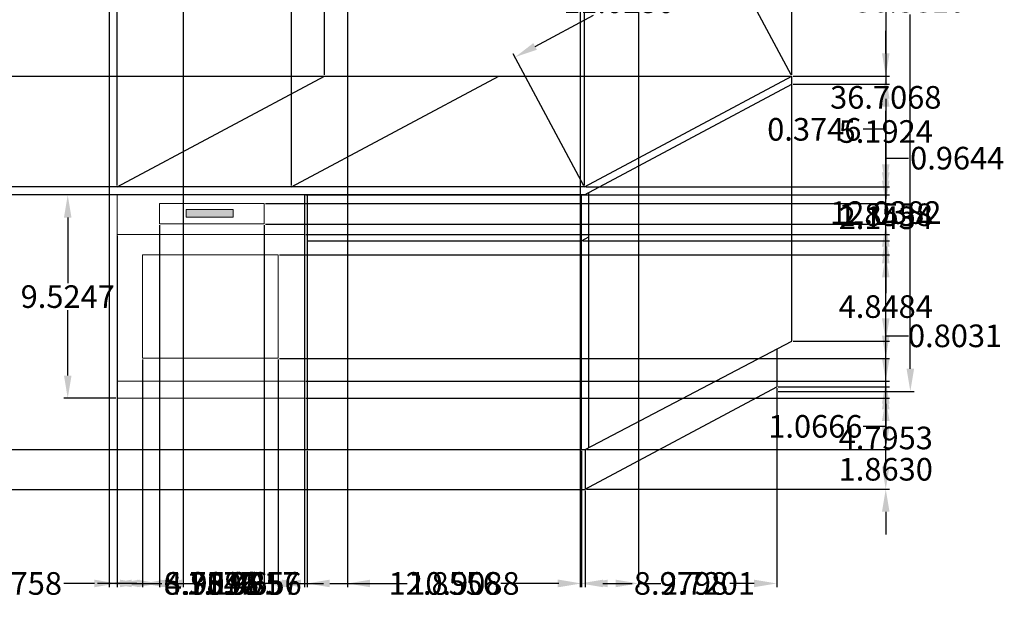
# Model space of a CAD drawing. Units: inches. Extents: x 32.3 to 119.3, y 11.9 to 64.
# Tile 2 of 3: x 73.2 to 119.3, y 11.9 to 39. Entities that reach past the tile are written whole.
import ezdxf

# ---------------------------------------------------------------- set-up
doc = ezdxf.new("R2010")
doc.units = ezdxf.units.IN
doc.header["$MEASUREMENT"] = 0
for name, color, linetype, lineweight in [('A-ANNO-DIMS', 2, 'Continuous', 18), ('A-EQPM', 4, 'Continuous', 18), ('A-EQPM-PATT', 8, 'Continuous', 13), ('A-FURN', 7, 'Continuous', 25)]:
    doc.layers.add(name, color=color, linetype=linetype, lineweight=lineweight)
doc.styles.get("Standard").update_dxf_attribs({"font": 'arial.ttf'})
doc.dimstyles.get("Standard").update_dxf_attribs({"dimtxt": 1.06, "dimasz": 1.06, "dimexe": 0.18, "dimexo": 0.0625, "dimgap": 0.09, "dimtad": 0, "dimtih": 1, "dimtoh": 1, "dimdec": 4, "dimzin": 0, "dimdsep": 46, "dimtxsty": 'Standard', "dimcen": 0.09, "dimadec": 0, "dimazin": 0, "dimtfac": 1, "dimtdec": 4, "dimtofl": 0, "dimtmove": 0, "dimatfit": 3, "dimfxl": 1, "dimtolj": 1, "dimtzin": 0, "dimarcsym": 0})

# ---------------------------------------------------------------- blocks, each defined once
blk = doc.blocks.new('*D8')
at = {"layer": 'A-ANNO-DIMS', "color": 0, "lineweight": -2, "transparency": 16777216}
for p, q in [((77.664, 30.769), (75.233, 30.769)), ((75.413, 29.709), (75.413, 26.637)), ((75.413, 22.304), (75.413, 25.375)), ((77.664, 21.244), (75.233, 21.244))]:
    blk.add_line(p, q, dxfattribs=at)
at = {"layer": 'A-ANNO-DIMS', "color": 0, "transparency": 16777216}
for points in [[(75.237, 29.709), (75.59, 29.709), (75.413, 30.769)], [(75.237, 22.304), (75.59, 22.304), (75.413, 21.244)]]:
    blk.add_solid(points, dxfattribs=at)
at = {"layer": 'Defpoints', "color": 0, "transparency": 16777216}
for p in [(75.413, 30.769), (77.726, 30.769), (77.726, 21.244)]:
    blk.add_point(p, dxfattribs=at)
at = {"layer": 'A-ANNO-DIMS', "color": 0, "transparency": 16777216, "insert": (75.413, 26.006), "char_height": 1.06, "attachment_point": 5}
blk.add_mtext('\\A1;9.5247', dxfattribs=at)
blk = doc.blocks.new('*D10')
at = {"layer": 'A-ANNO-DIMS', "color": 0, "lineweight": -2, "transparency": 16777216}
for p, q in [((109.325, 36.391), (106.022, 42.576)), ((105.172, 41.918), (102.428, 40.453)), ((97.318, 37.724), (100.062, 39.19)), ((99.602, 31.198), (96.298, 37.384))]:
    blk.add_line(p, q, dxfattribs=at)
at = {"layer": 'A-ANNO-DIMS', "color": 0, "transparency": 16777216}
for points in [[(105.088, 42.074), (105.255, 41.762), (106.107, 42.418)], [(97.235, 37.88), (97.401, 37.569), (96.383, 37.225)]]:
    blk.add_solid(points, dxfattribs=at)
at = {"layer": 'Defpoints', "color": 0, "transparency": 16777216}
for p in [(106.107, 42.418), (109.354, 36.335), (99.631, 31.143)]:
    blk.add_point(p, dxfattribs=at)
at = {"layer": 'A-ANNO-DIMS', "color": 0, "transparency": 16777216, "insert": (101.245, 39.821), "char_height": 1.06, "attachment_point": 5}
blk.add_mtext('\\A1;11.0230', dxfattribs=at)
blk = doc.blocks.new('*D11')
at = {"layer": 'A-ANNO-DIMS', "color": 0, "lineweight": -2, "transparency": 16777216}
for p, q in [((108.706, 58.146), (115.085, 58.146)), ((114.905, 57.086), (114.905, 40.487)), ((114.905, 22.625), (114.905, 39.223)), ((108.706, 21.565), (115.085, 21.565))]:
    blk.add_line(p, q, dxfattribs=at)
at = {"layer": 'A-ANNO-DIMS', "color": 0, "transparency": 16777216}
for points in [[(114.729, 57.086), (115.082, 57.086), (114.905, 58.146)], [(114.729, 22.625), (115.082, 22.625), (114.905, 21.565)]]:
    blk.add_solid(points, dxfattribs=at)
at = {"layer": 'Defpoints', "color": 0, "transparency": 16777216}
for p in [(108.644, 58.146), (114.905, 58.146), (108.644, 21.565)]:
    blk.add_point(p, dxfattribs=at)
at = {"layer": 'A-ANNO-DIMS', "color": 0, "transparency": 16777216, "insert": (114.905, 39.855), "char_height": 1.06, "attachment_point": 5}
blk.add_mtext('\\A1;36.5810', dxfattribs=at)
blk = doc.blocks.new('*D12')
at = {"layer": 'A-ANNO-DIMS', "color": 0, "lineweight": -2, "transparency": 16777216}
for p, q in [((42.508, 51.967), (42.508, 58.272)), ((109.354, 36.398), (109.354, 58.272)), ((43.568, 58.092), (73.222, 58.092)), ((108.294, 58.092), (78.64, 58.092))]:
    blk.add_line(p, q, dxfattribs=at)
at = {"layer": 'A-ANNO-DIMS', "color": 0, "transparency": 16777216}
for points in [[(43.568, 58.269), (43.568, 57.916), (42.508, 58.092)], [(108.294, 58.269), (108.294, 57.916), (109.354, 58.092)]]:
    blk.add_solid(points, dxfattribs=at)
at = {"layer": 'Defpoints', "color": 0, "transparency": 16777216}
for p in [(109.354, 58.092), (42.508, 51.905), (109.354, 36.335)]:
    blk.add_point(p, dxfattribs=at)
at = {"layer": 'A-ANNO-DIMS', "color": 0, "transparency": 16777216, "insert": (75.931, 58.092), "char_height": 1.06, "attachment_point": 5}
blk.add_mtext('\\A1;66.8465', dxfattribs=at)
blk = doc.blocks.new('*D16')
at = {"layer": 'A-ANNO-DIMS', "color": 0, "lineweight": -2, "transparency": 16777216}
for p, q in [((77.726, 21.181), (77.726, 12.388)), ((68.15, 18.786), (68.15, 12.388)), ((69.21, 12.568), (70.647, 12.568)), ((76.666, 12.568), (75.23, 12.568))]:
    blk.add_line(p, q, dxfattribs=at)
at = {"layer": 'A-ANNO-DIMS', "color": 0, "transparency": 16777216}
for points in [[(69.21, 12.745), (69.21, 12.391), (68.15, 12.568)], [(76.666, 12.745), (76.666, 12.391), (77.726, 12.568)]]:
    blk.add_solid(points, dxfattribs=at)
at = {"layer": 'Defpoints', "color": 0, "transparency": 16777216}
for p in [(77.726, 21.244), (68.15, 18.849), (77.726, 12.568)]:
    blk.add_point(p, dxfattribs=at)
at = {"layer": 'A-ANNO-DIMS', "color": 0, "transparency": 16777216, "insert": (72.938, 12.568), "char_height": 1.06, "attachment_point": 5}
blk.add_mtext('\\A1;9.5758', dxfattribs=at)
blk = doc.blocks.new('*D17')
at = {"layer": 'A-ANNO-DIMS', "color": 0, "lineweight": -2, "transparency": 16777216}
for p, q in [((77.726, 21.181), (77.726, 12.388)), ((86.511, 21.181), (86.511, 12.388)), ((78.786, 12.568), (79.828, 12.568)), ((85.451, 12.568), (84.409, 12.568))]:
    blk.add_line(p, q, dxfattribs=at)
at = {"layer": 'A-ANNO-DIMS', "color": 0, "transparency": 16777216}
for points in [[(78.786, 12.745), (78.786, 12.391), (77.726, 12.568)], [(85.451, 12.745), (85.451, 12.391), (86.511, 12.568)]]:
    blk.add_solid(points, dxfattribs=at)
at = {"layer": 'Defpoints', "color": 0, "transparency": 16777216}
for p in [(77.726, 21.244), (86.511, 21.244), (86.511, 12.568)]:
    blk.add_point(p, dxfattribs=at)
at = {"layer": 'A-ANNO-DIMS', "color": 0, "transparency": 16777216, "insert": (82.119, 12.568), "char_height": 1.06, "attachment_point": 5}
blk.add_mtext('\\A1;8.7846', dxfattribs=at)
blk = doc.blocks.new('*D18')
at = {"layer": 'A-ANNO-DIMS', "color": 0, "lineweight": -2, "transparency": 16777216}
for p, q in [((86.634, 18.786), (86.634, 12.388)), ((99.489, 18.786), (99.489, 12.388)), ((87.694, 12.568), (90.41, 12.568)), ((98.429, 12.568), (95.713, 12.568))]:
    blk.add_line(p, q, dxfattribs=at)
at = {"layer": 'A-ANNO-DIMS', "color": 0, "transparency": 16777216}
for points in [[(87.694, 12.745), (87.694, 12.391), (86.634, 12.568)], [(98.429, 12.745), (98.429, 12.391), (99.489, 12.568)]]:
    blk.add_solid(points, dxfattribs=at)
at = {"layer": 'Defpoints', "color": 0, "transparency": 16777216}
for p in [(86.634, 18.849), (99.489, 18.849), (99.489, 12.568)]:
    blk.add_point(p, dxfattribs=at)
at = {"layer": 'A-ANNO-DIMS', "color": 0, "transparency": 16777216, "insert": (93.062, 12.568), "char_height": 1.06, "attachment_point": 5}
blk.add_mtext('\\A1;12.8556', dxfattribs=at)
blk = doc.blocks.new('*D19')
at = {"layer": 'A-ANNO-DIMS', "color": 0, "lineweight": -2, "transparency": 16777216}
for p, q in [((108.644, 21.718), (108.644, 12.388)), ((99.664, 16.923), (99.664, 12.388)), ((100.724, 12.568), (101.862, 12.568)), ((107.584, 12.568), (106.446, 12.568))]:
    blk.add_line(p, q, dxfattribs=at)
at = {"layer": 'A-ANNO-DIMS', "color": 0, "transparency": 16777216}
for points in [[(100.724, 12.745), (100.724, 12.391), (99.664, 12.568)], [(107.584, 12.745), (107.584, 12.391), (108.644, 12.568)]]:
    blk.add_solid(points, dxfattribs=at)
at = {"layer": 'Defpoints', "color": 0, "transparency": 16777216}
for p in [(108.644, 21.781), (99.664, 16.986), (108.644, 12.568)]:
    blk.add_point(p, dxfattribs=at)
at = {"layer": 'A-ANNO-DIMS', "color": 0, "transparency": 16777216, "insert": (104.154, 12.568), "char_height": 1.06, "attachment_point": 5}
blk.add_mtext('\\A1;8.9798', dxfattribs=at)
blk = doc.blocks.new('*D20')
at = {"layer": 'A-ANNO-DIMS', "color": 0, "lineweight": -2, "transparency": 16777216}
for p, q in [((108.706, 21.781), (113.934, 21.781)), ((113.754, 20.721), (113.754, 20.015)), ((113.754, 18.046), (113.754, 18.752)), ((99.726, 16.986), (113.934, 16.986))]:
    blk.add_line(p, q, dxfattribs=at)
at = {"layer": 'A-ANNO-DIMS', "color": 0, "transparency": 16777216}
for points in [[(113.578, 20.721), (113.931, 20.721), (113.754, 21.781)], [(113.578, 18.046), (113.931, 18.046), (113.754, 16.986)]]:
    blk.add_solid(points, dxfattribs=at)
at = {"layer": 'Defpoints', "color": 0, "transparency": 16777216}
for p in [(108.644, 21.781), (113.754, 21.781), (99.664, 16.986)]:
    blk.add_point(p, dxfattribs=at)
at = {"layer": 'A-ANNO-DIMS', "color": 0, "transparency": 16777216, "insert": (113.754, 19.383), "char_height": 1.06, "attachment_point": 5}
blk.add_mtext('\\A1;4.7953', dxfattribs=at)
blk = doc.blocks.new('*D21')
at = {"layer": 'A-ANNO-DIMS', "color": 0, "lineweight": -2, "transparency": 16777216}
for p, q in [((113.754, 19.909), (113.754, 20.969)), ((99.727, 18.849), (113.934, 18.849)), ((99.726, 16.986), (113.934, 16.986)), ((113.754, 15.926), (113.754, 14.866))]:
    blk.add_line(p, q, dxfattribs=at)
at = {"layer": 'A-ANNO-DIMS', "color": 0, "transparency": 16777216}
for points in [[(113.578, 19.909), (113.931, 19.909), (113.754, 18.849)], [(113.578, 15.926), (113.931, 15.926), (113.754, 16.986)]]:
    blk.add_solid(points, dxfattribs=at)
at = {"layer": 'Defpoints', "color": 0, "transparency": 16777216}
for p in [(99.664, 18.849), (113.754, 18.849), (99.664, 16.986)]:
    blk.add_point(p, dxfattribs=at)
at = {"layer": 'A-ANNO-DIMS', "color": 0, "transparency": 16777216, "insert": (113.754, 17.917), "char_height": 1.06, "attachment_point": 5}
blk.add_mtext('\\A1;1.8630', dxfattribs=at)
blk = doc.blocks.new('*D22')
at = {"layer": 'A-ANNO-DIMS', "color": 0, "lineweight": -2, "transparency": 16777216}
for p, q in [((109.417, 35.961), (113.934, 35.961)), ((113.754, 34.901), (113.754, 30.573)), ((113.754, 24.983), (113.754, 29.31)), ((109.417, 23.923), (113.934, 23.923))]:
    blk.add_line(p, q, dxfattribs=at)
at = {"layer": 'A-ANNO-DIMS', "color": 0, "transparency": 16777216}
for points in [[(113.578, 34.901), (113.931, 34.901), (113.754, 35.961)], [(113.578, 24.983), (113.931, 24.983), (113.754, 23.923)]]:
    blk.add_solid(points, dxfattribs=at)
at = {"layer": 'Defpoints', "color": 0, "transparency": 16777216}
for p in [(109.354, 35.961), (113.754, 35.961), (109.354, 23.923)]:
    blk.add_point(p, dxfattribs=at)
at = {"layer": 'A-ANNO-DIMS', "color": 0, "transparency": 16777216, "insert": (113.754, 29.942), "char_height": 1.06, "attachment_point": 5}
blk.add_mtext('\\A1;12.0382', dxfattribs=at)
blk = doc.blocks.new('*D23')
at = {"layer": 'A-ANNO-DIMS', "color": 0, "lineweight": -2, "transparency": 16777216}
for p, q in [((102.22, 53.692), (113.934, 53.692)), ((113.754, 52.632), (113.754, 35.971)), ((113.754, 18.046), (113.754, 34.708)), ((99.726, 16.986), (113.934, 16.986))]:
    blk.add_line(p, q, dxfattribs=at)
at = {"layer": 'A-ANNO-DIMS', "color": 0, "transparency": 16777216}
for points in [[(113.578, 52.632), (113.931, 52.632), (113.754, 53.692)], [(113.578, 18.046), (113.931, 18.046), (113.754, 16.986)]]:
    blk.add_solid(points, dxfattribs=at)
at = {"layer": 'Defpoints', "color": 0, "transparency": 16777216}
for p in [(102.157, 53.692), (113.754, 53.692), (99.664, 16.986)]:
    blk.add_point(p, dxfattribs=at)
at = {"layer": 'A-ANNO-DIMS', "color": 0, "transparency": 16777216, "insert": (113.754, 35.339), "char_height": 1.06, "attachment_point": 5}
blk.add_mtext('\\A1;36.7068', dxfattribs=at)
blk = doc.blocks.new('*D27')
at = {"layer": 'A-ANNO-DIMS', "color": 0, "lineweight": -2, "transparency": 16777216}
for p, q in [((88.528, 44.465), (88.528, 12.388)), ((99.437, 44.465), (99.437, 12.388)), ((89.588, 12.568), (91.33, 12.568)), ((98.377, 12.568), (96.636, 12.568))]:
    blk.add_line(p, q, dxfattribs=at)
at = {"layer": 'A-ANNO-DIMS', "color": 0, "transparency": 16777216}
for points in [[(89.588, 12.745), (89.588, 12.391), (88.528, 12.568)], [(98.377, 12.745), (98.377, 12.391), (99.437, 12.568)]]:
    blk.add_solid(points, dxfattribs=at)
at = {"layer": 'Defpoints', "color": 0, "transparency": 16777216}
for p in [(88.528, 44.527), (99.437, 44.527), (99.437, 12.568)]:
    blk.add_point(p, dxfattribs=at)
at = {"layer": 'A-ANNO-DIMS', "color": 0, "transparency": 16777216, "insert": (93.983, 12.568), "char_height": 1.06, "attachment_point": 5}
blk.add_mtext('\\A1;10.9088', dxfattribs=at)
blk = doc.blocks.new('*D28')
at = {"layer": 'A-ANNO-DIMS', "color": 0, "lineweight": -2, "transparency": 16777216}
for p, q in [((102.157, 44.957), (102.157, 12.388)), ((99.437, 44.465), (99.437, 12.388)), ((100.497, 12.568), (101.097, 12.568)), ((102.157, 12.568), (103.217, 12.568))]:
    blk.add_line(p, q, dxfattribs=at)
at = {"layer": 'A-ANNO-DIMS', "color": 0, "transparency": 16777216}
for points in [[(100.497, 12.745), (100.497, 12.391), (99.437, 12.568)], [(101.097, 12.745), (101.097, 12.391), (102.157, 12.568)]]:
    blk.add_solid(points, dxfattribs=at)
at = {"layer": 'Defpoints', "color": 0, "transparency": 16777216}
for p in [(102.157, 45.02), (99.437, 44.527), (102.157, 12.568)]:
    blk.add_point(p, dxfattribs=at)
at = {"layer": 'A-ANNO-DIMS', "color": 0, "transparency": 16777216, "insert": (105.414, 12.568), "char_height": 1.06, "attachment_point": 5}
blk.add_mtext('\\A1;2.7201', dxfattribs=at)
blk = doc.blocks.new('*D33')
at = {"layer": 'A-ANNO-DIMS', "color": 0, "lineweight": -2, "transparency": 16777216}
for p, q in [((113.754, 31.829), (113.754, 32.889)), ((99.552, 30.769), (113.934, 30.769)), ((99.552, 28.625), (113.934, 28.625)), ((113.754, 27.565), (113.754, 26.505))]:
    blk.add_line(p, q, dxfattribs=at)
at = {"layer": 'A-ANNO-DIMS', "color": 0, "transparency": 16777216}
for points in [[(113.578, 31.829), (113.931, 31.829), (113.754, 30.769)], [(113.578, 27.565), (113.931, 27.565), (113.754, 28.625)]]:
    blk.add_solid(points, dxfattribs=at)
at = {"layer": 'Defpoints', "color": 0, "transparency": 16777216}
for p in [(99.489, 30.769), (113.754, 30.769), (99.489, 28.625)]:
    blk.add_point(p, dxfattribs=at)
at = {"layer": 'A-ANNO-DIMS', "color": 0, "transparency": 16777216, "insert": (113.754, 29.697), "char_height": 1.06, "attachment_point": 5}
blk.add_mtext('\\A1;2.1434', dxfattribs=at)
blk = doc.blocks.new('*D39')
at = {"layer": 'A-ANNO-DIMS', "color": 0, "lineweight": -2, "transparency": 16777216}
for p, q in [((77.355, 44.465), (77.355, 12.388)), ((80.821, 44.632), (80.821, 12.388)), ((78.415, 12.568), (79.761, 12.568)), ((80.821, 12.568), (81.881, 12.568))]:
    blk.add_line(p, q, dxfattribs=at)
at = {"layer": 'A-ANNO-DIMS', "color": 0, "transparency": 16777216}
for points in [[(78.415, 12.745), (78.415, 12.391), (77.355, 12.568)], [(79.761, 12.745), (79.761, 12.391), (80.821, 12.568)]]:
    blk.add_solid(points, dxfattribs=at)
at = {"layer": 'Defpoints', "color": 0, "transparency": 16777216}
for p in [(77.355, 44.527), (80.821, 44.694), (80.821, 12.568)]:
    blk.add_point(p, dxfattribs=at)
at = {"layer": 'A-ANNO-DIMS', "color": 0, "transparency": 16777216, "insert": (84.17, 12.568), "char_height": 1.06, "attachment_point": 5}
blk.add_mtext('\\A1;3.4656', dxfattribs=at)
blk = doc.blocks.new('*D45')
at = {"layer": 'A-ANNO-DIMS', "color": 0, "lineweight": -2, "transparency": 16777216}
for p, q in [((77.725, 31.206), (77.725, 58.272)), ((85.9, 31.206), (85.9, 58.272)), ((78.785, 58.092), (79.521, 58.092)), ((84.84, 58.092), (84.105, 58.092))]:
    blk.add_line(p, q, dxfattribs=at)
at = {"layer": 'A-ANNO-DIMS', "color": 0, "transparency": 16777216}
for points in [[(78.785, 58.269), (78.785, 57.916), (77.725, 58.092)], [(84.84, 58.269), (84.84, 57.916), (85.9, 58.092)]]:
    blk.add_solid(points, dxfattribs=at)
at = {"layer": 'Defpoints', "color": 0, "transparency": 16777216}
for p in [(85.9, 58.092), (77.725, 31.143), (85.9, 31.143)]:
    blk.add_point(p, dxfattribs=at)
at = {"layer": 'A-ANNO-DIMS', "color": 0, "transparency": 16777216, "insert": (81.813, 58.092), "char_height": 1.06, "attachment_point": 5}
blk.add_mtext('\\A1;8.1748', dxfattribs=at)
blk = doc.blocks.new('*D46')
at = {"layer": 'A-ANNO-DIMS', "color": 0, "lineweight": -2, "transparency": 16777216}
for p, q in [((77.725, 31.206), (77.725, 58.272)), ((87.449, 36.398), (87.449, 58.272)), ((78.785, 58.092), (80.293, 58.092)), ((86.389, 58.092), (84.881, 58.092))]:
    blk.add_line(p, q, dxfattribs=at)
at = {"layer": 'A-ANNO-DIMS', "color": 0, "transparency": 16777216}
for points in [[(78.785, 58.269), (78.785, 57.916), (77.725, 58.092)], [(86.389, 58.269), (86.389, 57.916), (87.449, 58.092)]]:
    blk.add_solid(points, dxfattribs=at)
at = {"layer": 'Defpoints', "color": 0, "transparency": 16777216}
for p in [(87.449, 58.092), (87.449, 36.335), (77.725, 31.143)]:
    blk.add_point(p, dxfattribs=at)
at = {"layer": 'A-ANNO-DIMS', "color": 0, "transparency": 16777216, "insert": (82.587, 58.092), "char_height": 1.06, "attachment_point": 5}
blk.add_mtext('\\A1;9.7235', dxfattribs=at)
blk = doc.blocks.new('*D47')
at = {"layer": 'A-ANNO-DIMS', "color": 0, "lineweight": -2, "transparency": 16777216}
for p, q in [((85.9, 31.206), (85.9, 58.272)), ((99.631, 31.206), (99.631, 58.272)), ((86.96, 58.092), (90.115, 58.092)), ((98.571, 58.092), (95.416, 58.092))]:
    blk.add_line(p, q, dxfattribs=at)
at = {"layer": 'A-ANNO-DIMS', "color": 0, "transparency": 16777216}
for points in [[(86.96, 58.269), (86.96, 57.916), (85.9, 58.092)], [(98.571, 58.269), (98.571, 57.916), (99.631, 58.092)]]:
    blk.add_solid(points, dxfattribs=at)
at = {"layer": 'Defpoints', "color": 0, "transparency": 16777216}
for p in [(99.631, 58.092), (85.9, 31.143), (99.631, 31.143)]:
    blk.add_point(p, dxfattribs=at)
at = {"layer": 'A-ANNO-DIMS', "color": 0, "transparency": 16777216, "insert": (92.765, 58.092), "char_height": 1.06, "attachment_point": 5}
blk.add_mtext('\\A1;13.7310', dxfattribs=at)
blk = doc.blocks.new('*D48')
at = {"layer": 'A-ANNO-DIMS', "color": 0, "lineweight": -2, "transparency": 16777216}
for p, q in [((99.631, 31.206), (99.631, 58.272)), ((109.354, 36.398), (109.354, 58.272)), ((100.691, 58.092), (102.198, 58.092)), ((108.294, 58.092), (106.787, 58.092))]:
    blk.add_line(p, q, dxfattribs=at)
at = {"layer": 'A-ANNO-DIMS', "color": 0, "transparency": 16777216}
for points in [[(100.691, 58.269), (100.691, 57.916), (99.631, 58.092)], [(108.294, 58.269), (108.294, 57.916), (109.354, 58.092)]]:
    blk.add_solid(points, dxfattribs=at)
at = {"layer": 'Defpoints', "color": 0, "transparency": 16777216}
for p in [(109.354, 58.092), (109.354, 36.335), (99.631, 31.143)]:
    blk.add_point(p, dxfattribs=at)
at = {"layer": 'A-ANNO-DIMS', "color": 0, "transparency": 16777216, "insert": (104.493, 58.092), "char_height": 1.06, "attachment_point": 5}
blk.add_mtext('\\A1;9.7235', dxfattribs=at)
blk = doc.blocks.new('*D49')
at = {"layer": 'A-ANNO-DIMS', "color": 0, "lineweight": -2, "transparency": 16777216}
for p, q in [((109.417, 36.335), (113.934, 36.335)), ((113.754, 35.275), (113.754, 34.37)), ((113.754, 32.203), (113.754, 33.108)), ((99.693, 31.143), (113.934, 31.143))]:
    blk.add_line(p, q, dxfattribs=at)
at = {"layer": 'A-ANNO-DIMS', "color": 0, "transparency": 16777216}
for points in [[(113.578, 35.275), (113.931, 35.275), (113.754, 36.335)], [(113.578, 32.203), (113.931, 32.203), (113.754, 31.143)]]:
    blk.add_solid(points, dxfattribs=at)
at = {"layer": 'Defpoints', "color": 0, "transparency": 16777216}
for p in [(109.354, 36.335), (113.754, 36.335), (99.631, 31.143)]:
    blk.add_point(p, dxfattribs=at)
at = {"layer": 'A-ANNO-DIMS', "color": 0, "transparency": 16777216, "insert": (113.754, 33.739), "char_height": 1.06, "attachment_point": 5}
blk.add_mtext('\\A1;5.1924', dxfattribs=at)
blk = doc.blocks.new('*D50')
at = {"layer": 'A-ANNO-DIMS', "color": 0, "lineweight": -2, "transparency": 16777216}
for p, q in [((113.754, 37.395), (113.754, 38.455)), ((109.417, 36.335), (113.934, 36.335)), ((109.417, 35.961), (113.934, 35.961)), ((113.754, 34.901), (113.754, 33.841)), ((113.754, 33.841), (112.694, 33.841))]:
    blk.add_line(p, q, dxfattribs=at)
at = {"layer": 'A-ANNO-DIMS', "color": 0, "transparency": 16777216}
for points in [[(113.578, 37.395), (113.931, 37.395), (113.754, 36.335)], [(113.578, 34.901), (113.931, 34.901), (113.754, 35.961)]]:
    blk.add_solid(points, dxfattribs=at)
at = {"layer": 'Defpoints', "color": 0, "transparency": 16777216}
for p in [(109.354, 36.335), (109.354, 35.961), (113.754, 35.961)]:
    blk.add_point(p, dxfattribs=at)
at = {"layer": 'A-ANNO-DIMS', "color": 0, "transparency": 16777216, "insert": (110.405, 33.841), "char_height": 1.06, "attachment_point": 5}
blk.add_mtext('\\A1;0.3746', dxfattribs=at)
blk = doc.blocks.new('*D52')
at = {"layer": 'A-ANNO-DIMS', "color": 0, "lineweight": -2, "transparency": 16777216}
for p, q in [((113.754, 31.829), (113.754, 32.889)), ((86.573, 30.769), (113.934, 30.769)), ((86.573, 28.913), (113.934, 28.913)), ((113.754, 27.853), (113.754, 26.793))]:
    blk.add_line(p, q, dxfattribs=at)
at = {"layer": 'A-ANNO-DIMS', "color": 0, "transparency": 16777216}
for points in [[(113.578, 31.829), (113.931, 31.829), (113.754, 30.769)], [(113.578, 27.853), (113.931, 27.853), (113.754, 28.913)]]:
    blk.add_solid(points, dxfattribs=at)
at = {"layer": 'Defpoints', "color": 0, "transparency": 16777216}
for p in [(86.511, 30.769), (113.754, 30.769), (86.511, 28.913)]:
    blk.add_point(p, dxfattribs=at)
at = {"layer": 'A-ANNO-DIMS', "color": 0, "transparency": 16777216, "insert": (113.754, 29.841), "char_height": 1.06, "attachment_point": 5}
blk.add_mtext('\\A1;1.8558', dxfattribs=at)
blk = doc.blocks.new('*D53')
at = {"layer": 'A-ANNO-DIMS', "color": 0, "lineweight": -2, "transparency": 16777216}
for p, q in [((113.754, 23.107), (113.754, 24.167)), ((113.754, 24.167), (114.814, 24.167)), ((86.573, 22.047), (113.934, 22.047)), ((86.573, 21.244), (113.934, 21.244)), ((113.754, 20.184), (113.754, 19.124))]:
    blk.add_line(p, q, dxfattribs=at)
at = {"layer": 'A-ANNO-DIMS', "color": 0, "transparency": 16777216}
for points in [[(113.578, 23.107), (113.931, 23.107), (113.754, 22.047)], [(113.578, 20.184), (113.931, 20.184), (113.754, 21.244)]]:
    blk.add_solid(points, dxfattribs=at)
at = {"layer": 'Defpoints', "color": 0, "transparency": 16777216}
for p in [(86.511, 22.047), (113.754, 22.047), (86.511, 21.244)]:
    blk.add_point(p, dxfattribs=at)
at = {"layer": 'A-ANNO-DIMS', "color": 0, "transparency": 16777216, "insert": (117.002, 24.167), "char_height": 1.06, "attachment_point": 5}
blk.add_mtext('\\A1;0.8031', dxfattribs=at)
blk = doc.blocks.new('*D54')
at = {"layer": 'A-ANNO-DIMS', "color": 0, "lineweight": -2, "transparency": 16777216}
for p, q in [((79.712, 29.344), (79.712, 12.388)), ((84.622, 29.344), (84.622, 12.388)), ((78.652, 12.568), (77.592, 12.568)), ((85.682, 12.568), (86.742, 12.568))]:
    blk.add_line(p, q, dxfattribs=at)
at = {"layer": 'A-ANNO-DIMS', "color": 0, "transparency": 16777216}
for points in [[(78.652, 12.745), (78.652, 12.391), (79.712, 12.568)], [(85.682, 12.745), (85.682, 12.391), (84.622, 12.568)]]:
    blk.add_solid(points, dxfattribs=at)
at = {"layer": 'Defpoints', "color": 0, "transparency": 16777216}
for p in [(79.712, 29.406), (84.622, 29.406), (84.622, 12.568)]:
    blk.add_point(p, dxfattribs=at)
at = {"layer": 'A-ANNO-DIMS', "color": 0, "transparency": 16777216, "insert": (82.167, 12.568), "char_height": 1.06, "attachment_point": 5}
blk.add_mtext('\\A1;4.9096', dxfattribs=at)
blk = doc.blocks.new('*D55')
at = {"layer": 'A-ANNO-DIMS', "color": 0, "lineweight": -2, "transparency": 16777216}
for p, q in [((113.754, 31.431), (113.754, 32.491)), ((113.754, 32.491), (114.814, 32.491)), ((84.684, 30.371), (113.934, 30.371)), ((84.684, 29.406), (113.934, 29.406)), ((113.754, 28.346), (113.754, 27.286))]:
    blk.add_line(p, q, dxfattribs=at)
at = {"layer": 'A-ANNO-DIMS', "color": 0, "transparency": 16777216}
for points in [[(113.578, 31.431), (113.931, 31.431), (113.754, 30.371)], [(113.578, 28.346), (113.931, 28.346), (113.754, 29.406)]]:
    blk.add_solid(points, dxfattribs=at)
at = {"layer": 'Defpoints', "color": 0, "transparency": 16777216}
for p in [(84.622, 30.371), (113.754, 30.371), (84.622, 29.406)]:
    blk.add_point(p, dxfattribs=at)
at = {"layer": 'A-ANNO-DIMS', "color": 0, "transparency": 16777216, "insert": (117.103, 32.491), "char_height": 1.06, "attachment_point": 5}
blk.add_mtext('\\A1;0.9644', dxfattribs=at)
blk = doc.blocks.new('*D56')
at = {"layer": 'A-ANNO-DIMS', "color": 0, "lineweight": -2, "transparency": 16777216}
for p, q in [((79.712, 29.344), (79.712, 12.388)), ((77.726, 28.85), (77.726, 12.388)), ((76.666, 12.568), (75.606, 12.568)), ((80.772, 12.568), (81.832, 12.568))]:
    blk.add_line(p, q, dxfattribs=at)
at = {"layer": 'A-ANNO-DIMS', "color": 0, "transparency": 16777216}
for points in [[(76.666, 12.745), (76.666, 12.391), (77.726, 12.568)], [(80.772, 12.745), (80.772, 12.391), (79.712, 12.568)]]:
    blk.add_solid(points, dxfattribs=at)
at = {"layer": 'Defpoints', "color": 0, "transparency": 16777216}
for p in [(79.712, 29.406), (77.726, 28.913), (79.712, 12.568)]:
    blk.add_point(p, dxfattribs=at)
at = {"layer": 'A-ANNO-DIMS', "color": 0, "transparency": 16777216, "insert": (84.072, 12.568), "char_height": 1.06, "attachment_point": 5}
blk.add_mtext('\\A1;1.9857', dxfattribs=at)
blk = doc.blocks.new('*D57')
at = {"layer": 'A-ANNO-DIMS', "color": 0, "lineweight": -2, "transparency": 16777216}
for p, q in [((78.925, 23.051), (78.925, 12.388)), ((85.283, 23.051), (85.283, 12.388)), ((77.865, 12.568), (76.805, 12.568)), ((86.343, 12.568), (87.403, 12.568))]:
    blk.add_line(p, q, dxfattribs=at)
at = {"layer": 'A-ANNO-DIMS', "color": 0, "transparency": 16777216}
for points in [[(77.865, 12.745), (77.865, 12.391), (78.925, 12.568)], [(86.343, 12.745), (86.343, 12.391), (85.283, 12.568)]]:
    blk.add_solid(points, dxfattribs=at)
at = {"layer": 'Defpoints', "color": 0, "transparency": 16777216}
for p in [(78.925, 23.113), (85.283, 23.113), (85.283, 12.568)]:
    blk.add_point(p, dxfattribs=at)
at = {"layer": 'A-ANNO-DIMS', "color": 0, "transparency": 16777216, "insert": (82.104, 12.568), "char_height": 1.06, "attachment_point": 5}
blk.add_mtext('\\A1;6.3577', dxfattribs=at)
blk = doc.blocks.new('*D58')
at = {"layer": 'A-ANNO-DIMS', "color": 0, "lineweight": -2, "transparency": 16777216}
for p, q in [((85.346, 27.962), (113.934, 27.962)), ((113.754, 26.902), (113.754, 26.169)), ((113.754, 24.173), (113.754, 24.906)), ((85.346, 23.113), (113.934, 23.113))]:
    blk.add_line(p, q, dxfattribs=at)
at = {"layer": 'A-ANNO-DIMS', "color": 0, "transparency": 16777216}
for points in [[(113.578, 26.902), (113.931, 26.902), (113.754, 27.962)], [(113.578, 24.173), (113.931, 24.173), (113.754, 23.113)]]:
    blk.add_solid(points, dxfattribs=at)
at = {"layer": 'Defpoints', "color": 0, "transparency": 16777216}
for p in [(85.283, 27.962), (113.754, 27.962), (85.283, 23.113)]:
    blk.add_point(p, dxfattribs=at)
at = {"layer": 'A-ANNO-DIMS', "color": 0, "transparency": 16777216, "insert": (113.754, 25.538), "char_height": 1.06, "attachment_point": 5}
blk.add_mtext('\\A1;4.8484', dxfattribs=at)
blk = doc.blocks.new('*D59')
at = {"layer": 'A-ANNO-DIMS', "color": 0, "lineweight": -2, "transparency": 16777216}
for p, q in [((78.925, 23.051), (78.925, 12.388)), ((77.726, 21.984), (77.726, 12.388)), ((76.666, 12.568), (75.606, 12.568)), ((79.985, 12.568), (81.045, 12.568))]:
    blk.add_line(p, q, dxfattribs=at)
at = {"layer": 'A-ANNO-DIMS', "color": 0, "transparency": 16777216}
for points in [[(76.666, 12.745), (76.666, 12.391), (77.726, 12.568)], [(79.985, 12.745), (79.985, 12.391), (78.925, 12.568)]]:
    blk.add_solid(points, dxfattribs=at)
at = {"layer": 'Defpoints', "color": 0, "transparency": 16777216}
for p in [(78.925, 23.113), (77.726, 22.047), (78.925, 12.568)]:
    blk.add_point(p, dxfattribs=at)
at = {"layer": 'A-ANNO-DIMS', "color": 0, "transparency": 16777216, "insert": (83.183, 12.568), "char_height": 1.06, "attachment_point": 5}
blk.add_mtext('\\A1;1.1991', dxfattribs=at)
blk = doc.blocks.new('*D60')
at = {"layer": 'A-ANNO-DIMS', "color": 0, "lineweight": -2, "transparency": 16777216}
for p, q in [((113.754, 24.173), (113.754, 25.233)), ((85.346, 23.113), (113.934, 23.113)), ((86.573, 22.047), (113.934, 22.047)), ((113.754, 20.987), (113.754, 19.927)), ((113.754, 19.927), (112.694, 19.927))]:
    blk.add_line(p, q, dxfattribs=at)
at = {"layer": 'A-ANNO-DIMS', "color": 0, "transparency": 16777216}
for points in [[(113.578, 24.173), (113.931, 24.173), (113.754, 23.113)], [(113.578, 20.987), (113.931, 20.987), (113.754, 22.047)]]:
    blk.add_solid(points, dxfattribs=at)
at = {"layer": 'Defpoints', "color": 0, "transparency": 16777216}
for p in [(85.283, 23.113), (86.511, 22.047), (113.754, 22.047)]:
    blk.add_point(p, dxfattribs=at)
at = {"layer": 'A-ANNO-DIMS', "color": 0, "transparency": 16777216, "insert": (110.454, 19.927), "char_height": 1.06, "attachment_point": 5}
blk.add_mtext('\\A1;1.0666', dxfattribs=at)

msp = doc.modelspace()

# ---------------------------------------------------------------- hatches: boundary and pattern name
at = {"layer": 'A-EQPM-PATT'}
h = msp.add_hatch(color=256, dxfattribs=at)
h.dxf.hatch_style = 1
h.paths.add_polyline_path([(83.17165, 30.07967), (80.9625, 30.07967), (80.9625, 29.73156), (83.17165, 29.73156)])

# ---------------------------------------------------------------- linework, layer by layer
at = {"layer": 'A-EQPM'}
for p, q in [((77.72624, 30.76852), (77.72624, 21.24379)), ((77.72624, 28.91269), (86.51084, 28.91269)), ((77.72624, 22.04688), (86.51084, 22.04688)), ((77.72624, 21.24379), (86.51084, 21.24379))]:
    msp.add_line(p, q, dxfattribs=at)
for points in [[(79.71198, 30.37063), (84.62155, 30.37063), (84.62155, 29.4062), (79.71198, 29.4062)], [(80.9625, 30.07967), (83.17165, 30.07967), (83.17165, 29.73156), (80.9625, 29.73156)], [(78.9253, 27.96182), (85.283, 27.96182), (85.283, 23.11347), (78.9253, 23.11347)]]:
    msp.add_lwpolyline(points, close=True, dxfattribs=at)
at = {"layer": 'A-FURN'}
for p, q in [((63.93986, 36.33549), (109.35445, 36.33549)), ((77.72517, 31.14308), (87.44863, 36.33549)), ((85.89998, 31.14308), (95.62344, 36.33549)), ((99.63098, 31.14308), (109.35445, 36.33549)), ((109.35445, 35.96092), (109.35445, 36.33549)), ((109.35445, 23.92276), (109.35445, 36.33549)), ((99.63098, 30.76852), (109.35445, 35.96092)), ((99.63098, 31.14308), (54.2164, 31.14308)), ((99.63098, 30.76852), (54.2164, 30.76852)), ((86.51084, 30.76852), (86.51084, 18.84862)), ((86.51084, 30.76852), (86.51084, 18.84862)), ((86.63388, 30.76852), (86.63388, 18.84862)), ((99.48949, 18.84862), (99.48949, 30.76852)), ((99.83435, 18.93781), (99.83435, 30.87712)), ((86.63388, 28.62511), (99.48949, 28.62511)), ((99.48949, 28.62511), (99.83435, 28.80597)), ((99.66402, 18.84862), (109.35445, 23.92276)), ((108.6437, 23.55059), (108.6437, 21.76878)), ((99.63098, 16.9681), (108.6437, 21.78096)), ((42.50795, 18.84862), (99.66402, 18.84862)), ((99.66402, 18.84862), (99.66386, 16.98565)), ((54.2164, 16.9681), (99.63098, 16.9681))]:
    msp.add_line(p, q, dxfattribs=at)

# ---------------------------------------------------------------- dimensions: what is measured, and where the dimension line sits
at = {"layer": 'A-ANNO-DIMS'}
for base, p1, p2, picture, middle in [((109.35445, 58.09249), (42.50795, 51.90451), (109.35445, 36.33549), '*D12', (75.9312, 58.09249)), ((85.89997, 58.09249), (77.72517, 31.14308), (85.89997, 31.14308), '*D45', (81.81257, 58.09249)), ((87.44863, 58.09249), (77.72517, 31.14308), (87.44863, 36.33549), '*D46', (82.5869, 58.09249)), ((99.63098, 58.09249), (85.89997, 31.14308), (99.63098, 31.14308), '*D47', (92.76548, 58.09249)), ((109.35445, 58.09249), (99.63098, 31.14308), (109.35445, 36.33549), '*D48', (104.49272, 58.09249)), ((102.15728, 12.5681), (99.43717, 44.52731), (102.15728, 45.01973), '*D28', (105.41427, 12.5681)), ((80.82094, 12.5681), (77.35538, 44.52731), (80.82094, 44.6944), '*D39', (84.17048, 12.5681)), ((99.43717, 12.5681), (88.52838, 44.52731), (99.43717, 44.52731), '*D27', (93.98277, 12.5681)), ((79.71198, 12.5681), (77.72624, 28.91269), (79.71198, 29.4062), '*D56', (84.07235, 12.5681)), ((84.62155, 12.5681), (79.71198, 29.4062), (84.62155, 29.4062), '*D54', (82.16677, 12.5681)), ((78.9253, 12.5681), (77.72624, 22.04688), (78.9253, 23.11347), '*D59', (83.18335, 12.5681)), ((85.283, 12.5681), (78.9253, 23.11347), (85.283, 23.11347), '*D57', (82.10415, 12.5681)), ((108.6437, 12.5681), (99.66386, 16.98566), (108.6437, 21.78096), '*D19', (104.15378, 12.5681)), ((77.72624, 12.5681), (68.15041, 18.84862), (77.72624, 21.24379), '*D16', (72.93832, 12.5681)), ((86.51084, 12.5681), (77.72624, 21.24379), (86.51084, 21.24379), '*D17', (82.11854, 12.5681)), ((99.48949, 12.5681), (86.63388, 18.84862), (99.48949, 18.84862), '*D18', (93.06168, 12.5681))]:
    dim = msp.add_linear_dim(base=base, p1=p1, p2=p2, dimstyle='Standard', override={"dimdec": 4, "dimlfac": 1, "dimrnd": 0, "dimzin": 0, "dimdsep": 46, "dimlunit": 2}, dxfattribs=at)
    dim.commit()
    dim.dimension.update_dxf_attribs({"geometry": picture, "text_midpoint": middle})
for base, p1, p2, override, picture, middle in [((114.90536, 58.14555), (108.6437, 21.56458), (108.6437, 58.14555), {"dimclrd": 0, "dimclre": 0, "dimclrt": 0}, '*D11', (114.90536, 39.85507)), ((113.75445, 53.69249), (99.66386, 16.98566), (102.15728, 53.69249), {"dimdec": 4, "dimlfac": 1, "dimrnd": 0, "dimzin": 0, "dimdsep": 46, "dimlunit": 2}, '*D23', (113.75445, 35.33907)), ((113.75445, 35.96092), (109.35445, 36.33549), (109.35445, 35.96092), {"dimdec": 4, "dimlfac": 1, "dimrnd": 0, "dimzin": 0, "dimdsep": 46, "dimlunit": 2}, '*D50', (110.40455, 33.84092)), ((113.75445, 36.33549), (99.63098, 31.14308), (109.35445, 36.33549), {"dimdec": 4, "dimlfac": 1, "dimrnd": 0, "dimzin": 0, "dimdsep": 46, "dimlunit": 2}, '*D49', (113.75445, 33.73929)), ((113.75445, 35.96092), (109.35445, 23.92276), (109.35445, 35.96092), {"dimdec": 4, "dimlfac": 1, "dimrnd": 0, "dimzin": 0, "dimdsep": 46, "dimlunit": 2}, '*D22', (113.75445, 29.94184)), ((113.75445, 30.37063), (84.62155, 29.4062), (84.62155, 30.37063), {"dimdec": 4, "dimlfac": 1, "dimrnd": 0, "dimzin": 0, "dimdsep": 46, "dimlunit": 2}, '*D55', (117.10254, 32.49063)), ((113.75445, 30.76852), (86.51084, 28.91269), (86.51084, 30.76852), {"dimdec": 4, "dimlfac": 1, "dimrnd": 0, "dimzin": 0, "dimdsep": 46, "dimlunit": 2}, '*D52', (113.75445, 29.8406)), ((113.75445, 30.76852), (99.48949, 28.62511), (99.48949, 30.76852), {"dimdec": 4, "dimlfac": 1, "dimrnd": 0, "dimzin": 0, "dimdsep": 46, "dimlunit": 2}, '*D33', (113.75445, 29.69682)), ((75.41334, 30.76852), (77.72624, 21.24379), (77.72624, 30.76852), {"dimclrd": 0, "dimclre": 0, "dimclrt": 0}, '*D8', (75.41334, 26.00615)), ((113.754446, 27.961824), (85.283003, 23.11347), (85.283003, 27.961824), {"dimdec": 4, "dimlfac": 1, "dimrnd": 0, "dimzin": 0, "dimdsep": 46, "dimlunit": 2}, '*D58', (113.754446, 25.537647)), ((113.75445, 22.04688), (85.283, 23.11347), (86.51084, 22.04688), {"dimdec": 4, "dimlfac": 1, "dimrnd": 0, "dimzin": 0, "dimdsep": 46, "dimlunit": 2}, '*D60', (110.45444, 19.92688)), ((113.75445, 22.04688), (86.51084, 21.24379), (86.51084, 22.04688), {"dimdec": 4, "dimlfac": 1, "dimrnd": 0, "dimzin": 0, "dimdsep": 46, "dimlunit": 2}, '*D53', (117.00239, 24.16688)), ((113.75445, 21.78096), (99.66386, 16.98566), (108.6437, 21.78096), {"dimdec": 4, "dimlfac": 1, "dimrnd": 0, "dimzin": 0, "dimdsep": 46, "dimlunit": 2}, '*D20', (113.75445, 19.38331)), ((113.75445, 18.84862), (99.66386, 16.98566), (99.66402, 18.84862), {"dimdec": 4, "dimlfac": 1, "dimrnd": 0, "dimzin": 0, "dimdsep": 46, "dimlunit": 2}, '*D21', (113.75445, 17.91714))]:
    dim = msp.add_linear_dim(base=base, p1=p1, p2=p2, angle=90, dimstyle='Standard', override=override, dxfattribs=at)
    dim.commit()
    dim.dimension.update_dxf_attribs({"geometry": picture, "text_midpoint": middle})
dim = msp.add_aligned_dim(p1=(99.63098, 31.14308), p2=(109.35445, 36.33549), distance=6.8949, dimstyle='Standard', override={"dimclrd": 0, "dimclre": 0, "dimclrt": 0}, dxfattribs=at)
dim.commit()
dim.dimension.update_dxf_attribs({"geometry": '*D10', "text_midpoint": (101.24486, 39.82132)})

doc.saveas('drawing.dxf')
